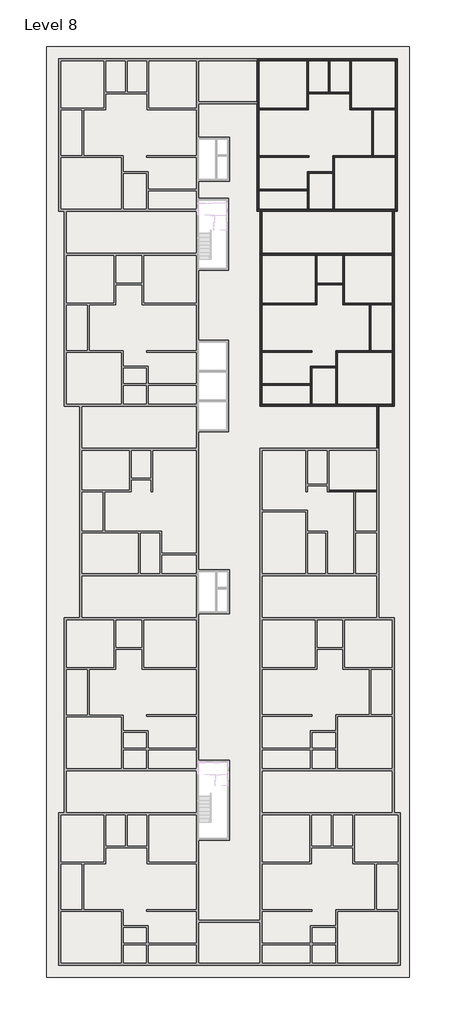
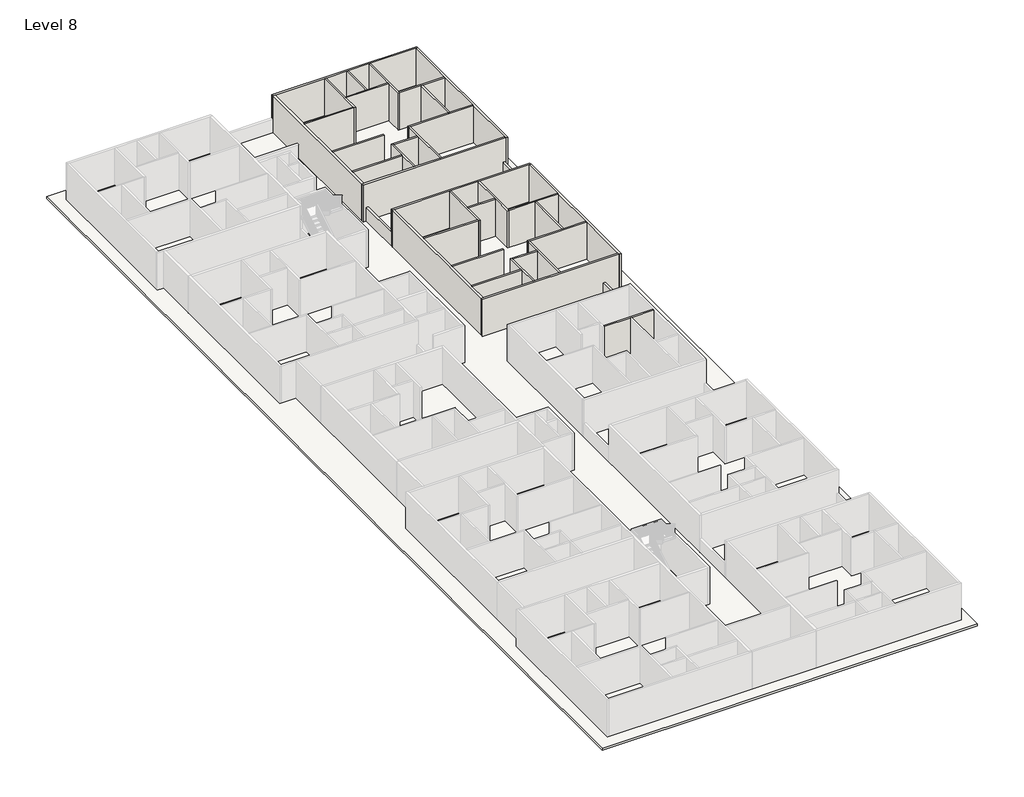
# One storey, part 4 of 8: 37 walls, 1 roof, 1 slab.
"""IFC4 building model written with IfcOpenShell, lengths in millimetres."""

from ifc_helpers import new_model, si_unit, frame, origin, place, context, project, spatial, polyline, outline, extrude, faceted_brep, element, save

model = new_model("IFC4")

# Units and contexts
model_context = context("Model", 3, world=origin())
ifc_project = project(units=[si_unit("LENGTHUNIT", "METRE", prefix="MILLI")], contexts=[model_context])

# Site, building, storey
site = spatial("IfcSite", under=ifc_project)
building = spatial("IfcBuilding", under=site)
storey = spatial("IfcBuildingStorey", under=building, Name="Level 8", Elevation=46570.6172466)

# Roof
placement = place(None, origin())
element("IfcRoof", 1, ObjectType="SLAB", at=placement, inside=storey, context=model_context, shape_type="SweptSolid", body=[
    extrude(outline(polyline([(-15237.9415084, -35021.5344126), (-15237.9415084, 36097.9216096), (12498.9443719, 36097.9216096), (12498.9443719, -35021.5344126), (-15237.9415084, -35021.5344126)]), holes=[polyline([(-3617.4415084, 29152.4900967), (-3617.4415084, 25799.6900967), (-1255.2415084, 25799.6900967), (-1255.2415084, 29152.4900967), (-3617.4415084, 29152.4900967)]), polyline([(-3617.4415084, 24490.1216096), (-3617.4415084, 19003.7216096), (-1331.4415084, 19003.7216096), (-1331.4415084, 24490.1216096), (-3617.4415084, 24490.1216096)]), polyline([(-3617.4415084, 13669.6303368), (-3617.4415084, 6659.2303368), (-1331.4415084, 6659.2303368), (-1331.4415084, 13669.6303368), (-3617.4415084, 13669.6303368)]), polyline([(-3617.4415084, -3882.2751812), (-3617.4415084, -7235.0751812), (-1255.2415084, -7235.0751812), (-1255.2415084, -3882.2751812), (-3617.4415084, -3882.2751812)]), polyline([(-3617.4415084, -18429.9851539), (-3617.4415084, -24525.9851539), (-1229.8415084, -24525.9851539), (-1229.8415084, -18429.9851539), (-3617.4415084, -18429.9851539)])]), frame((0.0, 0.0, 46570.6172466), z_axis=(0.0, 0.0, 1.0), x_axis=(1.0, 0.0, 0.0)), (0.0, 0.0, 1.0), 152.4),
])

# Slab
element("IfcSlab", 2, ObjectType="FLOOR", at=placement, inside=storey, context=model_context, shape_type="SweptSolid", body=[
    extrude(outline(polyline([(-14323.5415084, 35183.5216096), (11584.5443719, 35183.5216096), (11584.5443719, 23499.5216096), (11360.9214687, 23499.5216096), (11360.9214687, 8615.1216096), (10173.4714687, 8615.1216096), (10173.4714687, -7538.7344126), (11360.9214687, -7538.7344126), (11360.9214687, -22423.1344126), (11813.0584916, -22423.1344126), (11813.0584916, -34107.1344126), (11584.5443719, -34107.1344126), (-14323.5415084, -34107.1344126), (-14323.5415084, 35183.5216096)]), holes=[polyline([(-3617.4415084, 29152.4900967), (-3617.4415084, 25799.6900967), (-1255.2415084, 25799.6900967), (-1255.2415084, 29152.4900967), (-3617.4415084, 29152.4900967)]), polyline([(-3617.4415084, 24490.1216096), (-3617.4415084, 19003.7216096), (-1331.4415084, 19003.7216096), (-1331.4415084, 24490.1216096), (-3617.4415084, 24490.1216096)]), polyline([(-3617.4415084, 13669.6303368), (-3617.4415084, 6659.2303368), (-1331.4415084, 6659.2303368), (-1331.4415084, 13669.6303368), (-3617.4415084, 13669.6303368)]), polyline([(-3617.4415084, -3882.2751812), (-3617.4415084, -7235.0751812), (-1255.2415084, -7235.0751812), (-1255.2415084, -3882.2751812), (-3617.4415084, -3882.2751812)]), polyline([(-3617.4415084, -18429.9851539), (-3617.4415084, -24525.9851539), (-1229.8415084, -24525.9851539), (-1229.8415084, -18429.9851539), (-3617.4415084, -18429.9851539)])]), frame((0.0, 0.0, 45961.0172466), z_axis=(0.0, 0.0, 1.0), x_axis=(1.0, 0.0, 0.0)), (0.0, 0.0, 1.0), 609.6),
])

# Walls
element("IfcWall", 3, ObjectType="4.5\"", at=placement, inside=storey, context=model_context, shape_type="Brep", body=[
    faceted_brep([(6363.4714687, 2100.0216096, 46570.6172466), (8282.4584916, 2100.0216096, 46570.6172466), (8396.7584916, 2100.0216096, 46570.6172466), (10021.0714687, 2100.0216096, 46570.6172466), (10021.0714687, 2100.0216096, 49618.6172466), (8396.7584916, 2100.0216096, 49618.6172466), (8282.4584916, 2100.0216096, 49618.6172466), (6363.4714687, 2100.0216096, 49618.6172466), (6363.4714687, 2214.3216096, 46570.6172466), (6363.4714687, 2214.3216096, 49618.6172466), (10021.0714687, 2214.3216096, 49618.6172466), (10021.0714687, 2214.3216096, 46570.6172466)], [[[0, 1, 2, 3, 4, 5, 6, 7]], [[8, 9, 10, 11]], [[3, 2, 1, 0, 8, 11]], [[0, 7, 9, 8]], [[4, 3, 11, 10]], [[7, 6, 5, 4, 10, 9]]]),
])
element("IfcWall", 4, ObjectType="4.5\"", at=placement, inside=storey, context=model_context, shape_type="Brep", body=[
    faceted_brep([(5315.7214687, 20146.7216096, 46570.6172466), (5315.7214687, 16489.1216096, 46570.6172466), (5315.7214687, 16374.8216096, 46570.6172466), (5315.7214687, 16374.8216096, 49618.6172466), (5315.7214687, 16489.1216096, 49618.6172466), (5315.7214687, 20146.7216096, 49618.6172466), (5430.0214687, 20146.7216096, 46570.6172466), (5430.0214687, 20146.7216096, 49618.6172466), (5430.0214687, 18013.1216096, 49618.6172466), (5430.0214687, 17898.8216096, 49618.6172466), (5430.0214687, 16374.8216096, 49618.6172466), (5430.0214687, 16374.8216096, 46570.6172466), (5430.0214687, 17898.8216096, 46570.6172466), (5430.0214687, 18013.1216096, 46570.6172466)], [[[0, 1, 2, 3, 4, 5]], [[6, 7, 8, 9, 10, 11, 12, 13]], [[2, 1, 0, 6, 13, 12, 11]], [[0, 5, 7, 6]], [[3, 2, 11, 10]], [[5, 4, 3, 10, 9, 8, 7]]]),
])
element("IfcWall", 5, ObjectType="4.5\"", at=placement, inside=storey, context=model_context, shape_type="SweptSolid", body=[
    extrude(outline(polyline([(1259.3584916, 16489.1216096), (5315.7214687, 16489.1216096), (5315.7214687, 16374.8216096), (1259.3584916, 16374.8216096), (1259.3584916, 16489.1216096)])), frame((0.0, 0.0, 46570.6172466), z_axis=(0.0, 0.0, 1.0), x_axis=(1.0, 0.0, 0.0)), (0.0, 0.0, 1.0), 3048.0),
])
element("IfcWall", 6, ObjectType="4.5\"", at=placement, inside=storey, context=model_context, shape_type="SweptSolid", body=[
    extrude(outline(polyline([(7436.6214687, 17898.8216096), (5430.0214687, 17898.8216096), (5430.0214687, 18013.1216096), (7436.6214687, 18013.1216096), (7436.6214687, 17898.8216096)])), frame((0.0, 0.0, 46570.6172466), z_axis=(0.0, 0.0, 1.0), x_axis=(1.0, 0.0, 0.0)), (0.0, 0.0, 1.0), 3048.0),
])
element("IfcWall", 7, ObjectType="4.5\"", at=placement, inside=storey, context=model_context, shape_type="Brep", body=[
    faceted_brep([(7436.6214687, 20146.7216096, 46570.6172466), (7436.6214687, 18013.1216096, 46570.6172466), (7436.6214687, 17898.8216096, 46570.6172466), (7436.6214687, 16374.8216096, 46570.6172466), (7436.6214687, 16374.8216096, 49618.6172466), (7436.6214687, 17898.8216096, 49618.6172466), (7436.6214687, 18013.1216096, 49618.6172466), (7436.6214687, 20146.7216096, 49618.6172466), (7550.9214687, 20146.7216096, 46570.6172466), (7550.9214687, 20146.7216096, 49618.6172466), (7550.9214687, 16489.1216096, 49618.6172466), (7550.9214687, 16374.8216096, 49618.6172466), (7550.9214687, 16374.8216096, 46570.6172466), (7550.9214687, 16489.1216096, 46570.6172466)], [[[0, 1, 2, 3, 4, 5, 6, 7]], [[8, 9, 10, 11, 12, 13]], [[3, 2, 1, 0, 8, 13, 12]], [[0, 7, 9, 8]], [[4, 3, 12, 11]], [[7, 6, 5, 4, 11, 10, 9]]]),
])
element("IfcWall", 8, ObjectType="4.5\"", at=placement, inside=storey, context=model_context, shape_type="Brep", body=[
    faceted_brep([(7550.9214687, 16374.8216096, 46570.6172466), (9469.9084916, 16374.8216096, 46570.6172466), (9584.2084916, 16374.8216096, 46570.6172466), (11208.5214687, 16374.8216096, 46570.6172466), (11208.5214687, 16374.8216096, 49618.6172466), (9584.2084916, 16374.8216096, 49618.6172466), (9469.9084916, 16374.8216096, 49618.6172466), (7550.9214687, 16374.8216096, 49618.6172466), (7550.9214687, 16489.1216096, 46570.6172466), (7550.9214687, 16489.1216096, 49618.6172466), (11208.5214687, 16489.1216096, 49618.6172466), (11208.5214687, 16489.1216096, 46570.6172466)], [[[0, 1, 2, 3, 4, 5, 6, 7]], [[8, 9, 10, 11]], [[3, 2, 1, 0, 8, 11]], [[0, 7, 9, 8]], [[4, 3, 11, 10]], [[7, 6, 5, 4, 10, 9]]]),
])
element("IfcWall", 9, ObjectType="4.5\"", at=placement, inside=storey, context=model_context, shape_type="SweptSolid", body=[
    extrude(outline(polyline([(9469.9084916, 12869.6216096), (9469.9084916, 16374.8216096), (9584.2084916, 16374.8216096), (9584.2084916, 12869.6216096), (9469.9084916, 12869.6216096)])), frame((0.0, 0.0, 46570.6172466), z_axis=(0.0, 0.0, 1.0), x_axis=(1.0, 0.0, 0.0)), (0.0, 0.0, 1.0), 3048.0),
])
element("IfcWall", 10, ObjectType="4.5\"", at=placement, inside=storey, context=model_context, shape_type="Brep", body=[
    faceted_brep([(11208.5214687, 12869.6216096, 46570.6172466), (9584.2084916, 12869.6216096, 46570.6172466), (9469.9084916, 12869.6216096, 46570.6172466), (6885.4584916, 12869.6216096, 46570.6172466), (6885.4584916, 12869.6216096, 49618.6172466), (9469.9084916, 12869.6216096, 49618.6172466), (9584.2084916, 12869.6216096, 49618.6172466), (11208.5214687, 12869.6216096, 49618.6172466), (11208.5214687, 12755.3216096, 46570.6172466), (11208.5214687, 12755.3216096, 49618.6172466), (6999.7584916, 12755.3216096, 49618.6172466), (6885.4584916, 12755.3216096, 49618.6172466), (6885.4584916, 12755.3216096, 46570.6172466), (6999.7584916, 12755.3216096, 46570.6172466)], [[[0, 1, 2, 3, 4, 5, 6, 7]], [[8, 9, 10, 11, 12, 13]], [[3, 2, 1, 0, 8, 13, 12]], [[0, 7, 9, 8]], [[4, 3, 12, 11]], [[7, 6, 5, 4, 11, 10, 9]]]),
])
element("IfcWall", 11, ObjectType="4.5\"", at=placement, inside=storey, context=model_context, shape_type="Brep", body=[
    faceted_brep([(6885.4584916, 12755.3216096, 46570.6172466), (6885.4584916, 11663.1216096, 46570.6172466), (6885.4584916, 11548.8216096, 46570.6172466), (6885.4584916, 8767.5216096, 46570.6172466), (6885.4584916, 8767.5216096, 49618.6172466), (6885.4584916, 11548.8216096, 49618.6172466), (6885.4584916, 11663.1216096, 49618.6172466), (6885.4584916, 12755.3216096, 49618.6172466), (6999.7584916, 12755.3216096, 46570.6172466), (6999.7584916, 12755.3216096, 49618.6172466), (6999.7584916, 8767.5216096, 49618.6172466), (6999.7584916, 8767.5216096, 46570.6172466)], [[[0, 1, 2, 3, 4, 5, 6, 7]], [[8, 9, 10, 11]], [[3, 2, 1, 0, 8, 11]], [[0, 7, 9, 8]], [[4, 3, 11, 10]], [[7, 6, 5, 4, 10, 9]]]),
])
element("IfcWall", 12, ObjectType="4.5\"", at=placement, inside=storey, context=model_context, shape_type="Brep", body=[
    faceted_brep([(5056.6584916, 8767.5216096, 46570.6172466), (5056.6584916, 11548.8216096, 46570.6172466), (5056.6584916, 11663.1216096, 46570.6172466), (5056.6584916, 11663.1216096, 49618.6172466), (5056.6584916, 11548.8216096, 49618.6172466), (5056.6584916, 8767.5216096, 49618.6172466), (4942.3584916, 8767.5216096, 46570.6172466), (4942.3584916, 8767.5216096, 49618.6172466), (4942.3584916, 10215.3216096, 49618.6172466), (4942.3584916, 10329.6216096, 49618.6172466), (4942.3584916, 11663.1216096, 49618.6172466), (4942.3584916, 11663.1216096, 46570.6172466), (4942.3584916, 10329.6216096, 46570.6172466), (4942.3584916, 10215.3216096, 46570.6172466)], [[[0, 1, 2, 3, 4, 5]], [[6, 7, 8, 9, 10, 11, 12, 13]], [[2, 1, 0, 6, 13, 12, 11]], [[0, 5, 7, 6]], [[3, 2, 11, 10]], [[5, 4, 3, 10, 9, 8, 7]]]),
])
element("IfcWall", 13, ObjectType="4.5\"", at=placement, inside=storey, context=model_context, shape_type="SweptSolid", body=[
    extrude(outline(polyline([(6885.4584916, 11548.8216096), (5056.6584916, 11548.8216096), (5056.6584916, 11663.1216096), (6885.4584916, 11663.1216096), (6885.4584916, 11548.8216096)])), frame((0.0, 0.0, 46570.6172466), z_axis=(0.0, 0.0, 1.0), x_axis=(1.0, 0.0, 0.0)), (0.0, 0.0, 1.0), 3048.0),
])
element("IfcWall", 14, ObjectType="4.5\"", at=placement, inside=storey, context=model_context, shape_type="SweptSolid", body=[
    extrude(outline(polyline([(4942.3584916, 10215.3216096), (1259.3584916, 10215.3216096), (1259.3584916, 10329.6216096), (4942.3584916, 10329.6216096), (4942.3584916, 10215.3216096)])), frame((0.0, 0.0, 46570.6172466), z_axis=(0.0, 0.0, 1.0), x_axis=(1.0, 0.0, 0.0)), (0.0, 0.0, 1.0), 3048.0),
])
element("IfcWall", 15, ObjectType="4.5\"", at=placement, inside=storey, context=model_context, shape_type="SweptSolid", body=[
    extrude(outline(polyline([(5056.6584916, 12755.3216096), (1259.3584916, 12755.3216096), (1259.3584916, 12869.6216096), (5056.6584916, 12869.6216096), (5056.6584916, 12755.3216096)])), frame((0.0, 0.0, 46570.6172466), z_axis=(0.0, 0.0, 1.0), x_axis=(1.0, 0.0, 0.0)), (0.0, 0.0, 1.0), 3048.0),
])
element("IfcWall", 16, ObjectType="4.5\"", at=placement, inside=storey, context=model_context, shape_type="Brep", body=[
    faceted_brep([(4688.4443719, 35031.1216096, 46570.6172466), (4688.4443719, 31373.5216096, 46570.6172466), (4688.4443719, 31259.2216096, 46570.6172466), (4688.4443719, 31259.2216096, 49618.6172466), (4688.4443719, 31373.5216096, 49618.6172466), (4688.4443719, 35031.1216096, 49618.6172466), (4802.7443719, 35031.1216096, 46570.6172466), (4802.7443719, 35031.1216096, 49618.6172466), (4802.7443719, 32592.7216096, 49618.6172466), (4802.7443719, 32478.4216096, 49618.6172466), (4802.7443719, 31259.2216096, 49618.6172466), (4802.7443719, 31259.2216096, 46570.6172466), (4802.7443719, 32478.4216096, 46570.6172466), (4802.7443719, 32592.7216096, 46570.6172466)], [[[0, 1, 2, 3, 4, 5]], [[6, 7, 8, 9, 10, 11, 12, 13]], [[2, 1, 0, 6, 13, 12, 11]], [[0, 5, 7, 6]], [[3, 2, 11, 10]], [[5, 4, 3, 10, 9, 8, 7]]]),
])
element("IfcWall", 17, ObjectType="4.5\"", at=placement, inside=storey, context=model_context, shape_type="SweptSolid", body=[
    extrude(outline(polyline([(1030.8443719, 31373.5216096), (4688.4443719, 31373.5216096), (4688.4443719, 31259.2216096), (1030.8443719, 31259.2216096), (1030.8443719, 31373.5216096)])), frame((0.0, 0.0, 46570.6172466), z_axis=(0.0, 0.0, 1.0), x_axis=(1.0, 0.0, 0.0)), (0.0, 0.0, 1.0), 3048.0),
])
element("IfcWall", 18, ObjectType="4.5\"", at=placement, inside=storey, context=model_context, shape_type="Brep", body=[
    faceted_brep([(4802.7443719, 32478.4216096, 46570.6172466), (7965.0443719, 32478.4216096, 46570.6172466), (7965.0443719, 32478.4216096, 49618.6172466), (4802.7443719, 32478.4216096, 49618.6172466), (4802.7443719, 32592.7216096, 46570.6172466), (4802.7443719, 32592.7216096, 49618.6172466), (6326.7443719, 32592.7216096, 49618.6172466), (6441.0443719, 32592.7216096, 49618.6172466), (7965.0443719, 32592.7216096, 49618.6172466), (7965.0443719, 32592.7216096, 46570.6172466), (6441.0443719, 32592.7216096, 46570.6172466), (6326.7443719, 32592.7216096, 46570.6172466)], [[[0, 1, 2, 3]], [[4, 5, 6, 7, 8, 9, 10, 11]], [[1, 0, 4, 11, 10, 9]], [[0, 3, 5, 4]], [[2, 1, 9, 8]], [[3, 2, 8, 7, 6, 5]]]),
])
element("IfcWall", 19, ObjectType="4.5\"", at=placement, inside=storey, context=model_context, shape_type="SweptSolid", body=[
    extrude(outline(polyline([(6326.7443719, 32592.7216096), (6326.7443719, 35031.1216096), (6441.0443719, 35031.1216096), (6441.0443719, 32592.7216096), (6326.7443719, 32592.7216096)])), frame((0.0, 0.0, 46570.6172466), z_axis=(0.0, 0.0, 1.0), x_axis=(1.0, 0.0, 0.0)), (0.0, 0.0, 1.0), 3048.0),
])
element("IfcWall", 20, ObjectType="4.5\"", at=placement, inside=storey, context=model_context, shape_type="Brep", body=[
    faceted_brep([(7965.0443719, 35031.1216096, 46570.6172466), (7965.0443719, 32592.7216096, 46570.6172466), (7965.0443719, 32478.4216096, 46570.6172466), (7965.0443719, 31259.2216096, 46570.6172466), (7965.0443719, 31259.2216096, 49618.6172466), (7965.0443719, 32478.4216096, 49618.6172466), (7965.0443719, 32592.7216096, 49618.6172466), (7965.0443719, 35031.1216096, 49618.6172466), (8079.3443719, 35031.1216096, 46570.6172466), (8079.3443719, 35031.1216096, 49618.6172466), (8079.3443719, 31373.5216096, 49618.6172466), (8079.3443719, 31259.2216096, 49618.6172466), (8079.3443719, 31259.2216096, 46570.6172466), (8079.3443719, 31373.5216096, 46570.6172466)], [[[0, 1, 2, 3, 4, 5, 6, 7]], [[8, 9, 10, 11, 12, 13]], [[3, 2, 1, 0, 8, 13, 12]], [[0, 7, 9, 8]], [[4, 3, 12, 11]], [[7, 6, 5, 4, 11, 10, 9]]]),
])
element("IfcWall", 21, ObjectType="4.5\"", at=placement, inside=storey, context=model_context, shape_type="Brep", body=[
    faceted_brep([(8079.3443719, 31259.2216096, 46570.6172466), (9641.4443719, 31259.2216096, 46570.6172466), (9755.7443719, 31259.2216096, 46570.6172466), (11432.1443719, 31259.2216096, 46570.6172466), (11432.1443719, 31259.2216096, 49618.6172466), (9755.7443719, 31259.2216096, 49618.6172466), (9641.4443719, 31259.2216096, 49618.6172466), (8079.3443719, 31259.2216096, 49618.6172466), (8079.3443719, 31373.5216096, 46570.6172466), (8079.3443719, 31373.5216096, 49618.6172466), (11432.1443719, 31373.5216096, 49618.6172466), (11432.1443719, 31373.5216096, 46570.6172466)], [[[0, 1, 2, 3, 4, 5, 6, 7]], [[8, 9, 10, 11]], [[3, 2, 1, 0, 8, 11]], [[0, 7, 9, 8]], [[4, 3, 11, 10]], [[7, 6, 5, 4, 10, 9]]]),
])
element("IfcWall", 22, ObjectType="4.5\"", at=placement, inside=storey, context=model_context, shape_type="SweptSolid", body=[
    extrude(outline(polyline([(9641.4443719, 27754.0216096), (9641.4443719, 31259.2216096), (9755.7443719, 31259.2216096), (9755.7443719, 27754.0216096), (9641.4443719, 27754.0216096)])), frame((0.0, 0.0, 46570.6172466), z_axis=(0.0, 0.0, 1.0), x_axis=(1.0, 0.0, 0.0)), (0.0, 0.0, 1.0), 3048.0),
])
element("IfcWall", 23, ObjectType="4.5\"", at=placement, inside=storey, context=model_context, shape_type="Brep", body=[
    faceted_brep([(11432.1443719, 27754.0216096, 46570.6172466), (9755.7443719, 27754.0216096, 46570.6172466), (9641.4443719, 27754.0216096, 46570.6172466), (6656.9443719, 27754.0216096, 46570.6172466), (6656.9443719, 27754.0216096, 49618.6172466), (9641.4443719, 27754.0216096, 49618.6172466), (9755.7443719, 27754.0216096, 49618.6172466), (11432.1443719, 27754.0216096, 49618.6172466), (11432.1443719, 27639.7216096, 46570.6172466), (11432.1443719, 27639.7216096, 49618.6172466), (6771.2443719, 27639.7216096, 49618.6172466), (6656.9443719, 27639.7216096, 49618.6172466), (6656.9443719, 27639.7216096, 46570.6172466), (6771.2443719, 27639.7216096, 46570.6172466)], [[[0, 1, 2, 3, 4, 5, 6, 7]], [[8, 9, 10, 11, 12, 13]], [[3, 2, 1, 0, 8, 13, 12]], [[0, 7, 9, 8]], [[4, 3, 12, 11]], [[7, 6, 5, 4, 11, 10, 9]]]),
])
element("IfcWall", 24, ObjectType="4.5\"", at=placement, inside=storey, context=model_context, shape_type="Brep", body=[
    faceted_brep([(6656.9443719, 27639.7216096, 46570.6172466), (6656.9443719, 26547.5216096, 46570.6172466), (6656.9443719, 26433.2216096, 46570.6172466), (6656.9443719, 23651.9216096, 46570.6172466), (6656.9443719, 23651.9216096, 49618.6172466), (6656.9443719, 26433.2216096, 49618.6172466), (6656.9443719, 26547.5216096, 49618.6172466), (6656.9443719, 27639.7216096, 49618.6172466), (6771.2443719, 27639.7216096, 46570.6172466), (6771.2443719, 27639.7216096, 49618.6172466), (6771.2443719, 23651.9216096, 49618.6172466), (6771.2443719, 23651.9216096, 46570.6172466)], [[[0, 1, 2, 3, 4, 5, 6, 7]], [[8, 9, 10, 11]], [[3, 2, 1, 0, 8, 11]], [[0, 7, 9, 8]], [[4, 3, 11, 10]], [[7, 6, 5, 4, 10, 9]]]),
])
element("IfcWall", 25, ObjectType="4.5\"", at=placement, inside=storey, context=model_context, shape_type="SweptSolid", body=[
    extrude(outline(polyline([(4713.8443719, 25099.7216096), (1030.8443719, 25099.7216096), (1030.8443719, 25214.0216096), (4713.8443719, 25214.0216096), (4713.8443719, 25099.7216096)])), frame((0.0, 0.0, 46570.6172466), z_axis=(0.0, 0.0, 1.0), x_axis=(1.0, 0.0, 0.0)), (0.0, 0.0, 1.0), 3048.0),
])
element("IfcWall", 26, ObjectType="4.5\"", at=placement, inside=storey, context=model_context, shape_type="Brep", body=[
    faceted_brep([(4828.1443719, 23651.9216096, 46570.6172466), (4828.1443719, 26433.2216096, 46570.6172466), (4828.1443719, 26547.5216096, 46570.6172466), (4828.1443719, 26547.5216096, 49618.6172466), (4828.1443719, 26433.2216096, 49618.6172466), (4828.1443719, 23651.9216096, 49618.6172466), (4713.8443719, 23651.9216096, 46570.6172466), (4713.8443719, 23651.9216096, 49618.6172466), (4713.8443719, 25099.7216096, 49618.6172466), (4713.8443719, 25214.0216096, 49618.6172466), (4713.8443719, 26547.5216096, 49618.6172466), (4713.8443719, 26547.5216096, 46570.6172466), (4713.8443719, 25214.0216096, 46570.6172466), (4713.8443719, 25099.7216096, 46570.6172466)], [[[0, 1, 2, 3, 4, 5]], [[6, 7, 8, 9, 10, 11, 12, 13]], [[2, 1, 0, 6, 13, 12, 11]], [[0, 5, 7, 6]], [[3, 2, 11, 10]], [[5, 4, 3, 10, 9, 8, 7]]]),
])
element("IfcWall", 27, ObjectType="4.5\"", at=placement, inside=storey, context=model_context, shape_type="SweptSolid", body=[
    extrude(outline(polyline([(6656.9443719, 26433.2216096), (4828.1443719, 26433.2216096), (4828.1443719, 26547.5216096), (6656.9443719, 26547.5216096), (6656.9443719, 26433.2216096)])), frame((0.0, 0.0, 46570.6172466), z_axis=(0.0, 0.0, 1.0), x_axis=(1.0, 0.0, 0.0)), (0.0, 0.0, 1.0), 3048.0),
])
element("IfcWall", 28, ObjectType="4.5\"", at=placement, inside=storey, context=model_context, shape_type="SweptSolid", body=[
    extrude(outline(polyline([(4828.1443719, 27639.7216096), (1030.8443719, 27639.7216096), (1030.8443719, 27754.0216096), (4828.1443719, 27754.0216096), (4828.1443719, 27639.7216096)])), frame((0.0, 0.0, 46570.6172466), z_axis=(0.0, 0.0, 1.0), x_axis=(1.0, 0.0, 0.0)), (0.0, 0.0, 1.0), 3048.0),
])
element("IfcWall", 29, ObjectType="6\"", at=placement, inside=storey, context=model_context, shape_type="Brep", body=[
    faceted_brep([(1106.9584916, 20146.7216096, 49618.6172466), (1106.9584916, 20146.7216096, 46570.6172466), (1259.3584916, 20146.7216096, 46570.6172466), (5315.7214687, 20146.7216096, 46570.6172466), (5430.0214687, 20146.7216096, 46570.6172466), (7436.6214687, 20146.7216096, 46570.6172466), (7550.9214687, 20146.7216096, 46570.6172466), (11208.5214687, 20146.7216096, 46570.6172466), (11360.9214687, 20146.7216096, 46570.6172466), (11360.9214687, 20146.7216096, 49618.6172466), (11208.5214687, 20146.7216096, 49618.6172466), (7550.9214687, 20146.7216096, 49618.6172466), (7436.6214687, 20146.7216096, 49618.6172466), (5430.0214687, 20146.7216096, 49618.6172466), (5315.7214687, 20146.7216096, 49618.6172466), (1259.3584916, 20146.7216096, 49618.6172466), (1106.9584916, 20299.1216096, 46570.6172466), (1106.9584916, 20299.1216096, 47789.8172466), (1106.9584916, 20299.1216096, 49618.6172466), (11360.9214687, 20299.1216096, 49618.6172466), (11360.9214687, 20299.1216096, 47789.8172466), (11360.9214687, 20299.1216096, 46570.6172466), (11208.5214687, 20299.1216096, 46570.6172466), (1259.3584916, 20299.1216096, 46570.6172466)], [[[0, 1, 2, 3, 4, 5, 6, 7, 8, 9, 10, 11, 12, 13, 14, 15]], [[16, 17, 18, 19, 20, 21, 22, 23]], [[8, 7, 6, 5, 4, 3, 2, 1, 16, 23, 22, 21]], [[0, 18, 17, 16, 1]], [[8, 21, 20, 19, 9]], [[0, 15, 14, 13, 12, 11, 10, 9, 19, 18]]]),
])
element("IfcWall", 30, ObjectType="6\"", at=placement, inside=storey, context=model_context, shape_type="Brep", body=[
    faceted_brep([(11208.5214687, 20146.7216096, 49618.6172466), (11208.5214687, 20146.7216096, 46570.6172466), (11208.5214687, 16489.1216096, 46570.6172466), (11208.5214687, 16374.8216096, 46570.6172466), (11208.5214687, 12869.6216096, 46570.6172466), (11208.5214687, 12755.3216096, 46570.6172466), (11208.5214687, 8767.5216096, 46570.6172466), (11208.5214687, 8615.1216096, 46570.6172466), (11208.5214687, 8615.1216096, 49618.6172466), (11208.5214687, 8767.5216096, 49618.6172466), (11208.5214687, 12755.3216096, 49618.6172466), (11208.5214687, 12869.6216096, 49618.6172466), (11208.5214687, 16374.8216096, 49618.6172466), (11208.5214687, 16489.1216096, 49618.6172466), (11360.9214687, 20146.7216096, 46570.6172466), (11360.9214687, 20146.7216096, 49618.6172466), (11360.9214687, 8615.1216096, 49618.6172466), (11360.9214687, 8615.1216096, 46570.6172466)], [[[0, 1, 2, 3, 4, 5, 6, 7, 8, 9, 10, 11, 12, 13]], [[14, 15, 16, 17]], [[7, 6, 5, 4, 3, 2, 1, 14, 17]], [[8, 7, 17, 16]], [[0, 15, 14, 1]], [[0, 13, 12, 11, 10, 9, 8, 16, 15]]]),
])
element("IfcWall", 31, ObjectType="6\"", at=placement, inside=storey, context=model_context, shape_type="Brep", body=[
    faceted_brep([(11208.5214687, 8767.5216096, 46570.6172466), (6999.7584916, 8767.5216096, 46570.6172466), (6885.4584916, 8767.5216096, 46570.6172466), (5056.6584916, 8767.5216096, 46570.6172466), (4942.3584916, 8767.5216096, 46570.6172466), (1259.3584916, 8767.5216096, 46570.6172466), (1106.9584916, 8767.5216096, 46570.6172466), (1106.9584916, 8767.5216096, 49618.6172466), (1259.3584916, 8767.5216096, 49618.6172466), (4942.3584916, 8767.5216096, 49618.6172466), (5056.6584916, 8767.5216096, 49618.6172466), (6885.4584916, 8767.5216096, 49618.6172466), (6999.7584916, 8767.5216096, 49618.6172466), (11208.5214687, 8767.5216096, 49618.6172466), (11208.5214687, 8615.1216096, 46570.6172466), (11208.5214687, 8615.1216096, 49618.6172466), (1106.9584916, 8615.1216096, 49618.6172466), (1106.9584916, 8615.1216096, 46570.6172466), (10021.0714687, 8615.1216096, 46570.6172466), (10173.4714687, 8615.1216096, 46570.6172466)], [[[0, 1, 2, 3, 4, 5, 6, 7, 8, 9, 10, 11, 12, 13]], [[14, 15, 16, 17, 18, 19]], [[6, 5, 4, 3, 2, 1, 0, 14, 19, 18, 17]], [[0, 13, 15, 14]], [[7, 6, 17, 16]], [[13, 12, 11, 10, 9, 8, 7, 16, 15]]]),
])
element("IfcWall", 32, ObjectType="6\"", at=placement, inside=storey, context=model_context, shape_type="Brep", body=[
    faceted_brep([(1259.3584916, 8767.5216096, 46570.6172466), (1259.3584916, 10215.3216096, 46570.6172466), (1259.3584916, 10329.6216096, 46570.6172466), (1259.3584916, 12755.3216096, 46570.6172466), (1259.3584916, 12869.6216096, 46570.6172466), (1259.3584916, 16374.8216096, 46570.6172466), (1259.3584916, 16489.1216096, 46570.6172466), (1259.3584916, 20146.7216096, 46570.6172466), (1259.3584916, 20146.7216096, 49618.6172466), (1259.3584916, 16489.1216096, 49618.6172466), (1259.3584916, 16374.8216096, 49618.6172466), (1259.3584916, 12869.6216096, 49618.6172466), (1259.3584916, 12755.3216096, 49618.6172466), (1259.3584916, 10329.6216096, 49618.6172466), (1259.3584916, 10215.3216096, 49618.6172466), (1259.3584916, 8767.5216096, 49618.6172466), (1106.9584916, 8767.5216096, 46570.6172466), (1106.9584916, 8767.5216096, 49618.6172466), (1106.9584916, 20146.7216096, 49618.6172466), (1106.9584916, 20146.7216096, 46570.6172466)], [[[0, 1, 2, 3, 4, 5, 6, 7, 8, 9, 10, 11, 12, 13, 14, 15]], [[16, 17, 18, 19]], [[7, 6, 5, 4, 3, 2, 1, 0, 16, 19]], [[0, 15, 17, 16]], [[7, 19, 18, 8]], [[15, 14, 13, 12, 11, 10, 9, 8, 18, 17]]]),
])
element("IfcWall", 33, ObjectType="6\"", at=placement, inside=storey, context=model_context, shape_type="Brep", body=[
    faceted_brep([(878.4443719, 35031.1216096, 49618.6172466), (878.4443719, 35031.1216096, 46570.6172466), (1030.8443719, 35031.1216096, 46570.6172466), (4688.4443719, 35031.1216096, 46570.6172466), (4802.7443719, 35031.1216096, 46570.6172466), (6326.7443719, 35031.1216096, 46570.6172466), (6441.0443719, 35031.1216096, 46570.6172466), (7965.0443719, 35031.1216096, 46570.6172466), (8079.3443719, 35031.1216096, 46570.6172466), (11432.1443719, 35031.1216096, 46570.6172466), (11584.5443719, 35031.1216096, 46570.6172466), (11584.5443719, 35031.1216096, 49618.6172466), (11432.1443719, 35031.1216096, 49618.6172466), (8079.3443719, 35031.1216096, 49618.6172466), (7965.0443719, 35031.1216096, 49618.6172466), (6441.0443719, 35031.1216096, 49618.6172466), (6326.7443719, 35031.1216096, 49618.6172466), (4802.7443719, 35031.1216096, 49618.6172466), (4688.4443719, 35031.1216096, 49618.6172466), (1030.8443719, 35031.1216096, 49618.6172466), (878.4443719, 35183.5216096, 46570.6172466), (878.4443719, 35183.5216096, 49618.6172466), (11584.5443719, 35183.5216096, 49618.6172466), (11584.5443719, 35183.5216096, 46570.6172466)], [[[0, 1, 2, 3, 4, 5, 6, 7, 8, 9, 10, 11, 12, 13, 14, 15, 16, 17, 18, 19]], [[20, 21, 22, 23]], [[10, 9, 8, 7, 6, 5, 4, 3, 2, 1, 20, 23]], [[11, 10, 23, 22]], [[0, 21, 20, 1]], [[0, 19, 18, 17, 16, 15, 14, 13, 12, 11, 22, 21]]]),
])
element("IfcWall", 34, ObjectType="6\"", at=placement, inside=storey, context=model_context, shape_type="Brep", body=[
    faceted_brep([(11432.1443719, 35031.1216096, 46570.6172466), (11432.1443719, 31373.5216096, 46570.6172466), (11432.1443719, 31259.2216096, 46570.6172466), (11432.1443719, 27754.0216096, 46570.6172466), (11432.1443719, 27639.7216096, 46570.6172466), (11432.1443719, 23651.9216096, 46570.6172466), (11432.1443719, 23499.5216096, 46570.6172466), (11432.1443719, 23499.5216096, 49618.6172466), (11432.1443719, 23651.9216096, 49618.6172466), (11432.1443719, 27639.7216096, 49618.6172466), (11432.1443719, 27754.0216096, 49618.6172466), (11432.1443719, 31259.2216096, 49618.6172466), (11432.1443719, 31373.5216096, 49618.6172466), (11432.1443719, 35031.1216096, 49618.6172466), (11584.5443719, 35031.1216096, 46570.6172466), (11584.5443719, 35031.1216096, 49618.6172466), (11584.5443719, 23499.5216096, 49618.6172466), (11584.5443719, 23499.5216096, 46570.6172466)], [[[0, 1, 2, 3, 4, 5, 6, 7, 8, 9, 10, 11, 12, 13]], [[14, 15, 16, 17]], [[6, 5, 4, 3, 2, 1, 0, 14, 17]], [[0, 13, 15, 14]], [[7, 6, 17, 16]], [[13, 12, 11, 10, 9, 8, 7, 16, 15]]]),
])
element("IfcWall", 35, ObjectType="6\"", at=placement, inside=storey, context=model_context, shape_type="Brep", body=[
    faceted_brep([(11432.1443719, 23651.9216096, 46570.6172466), (6771.2443719, 23651.9216096, 46570.6172466), (6656.9443719, 23651.9216096, 46570.6172466), (4828.1443719, 23651.9216096, 46570.6172466), (4713.8443719, 23651.9216096, 46570.6172466), (1030.8443719, 23651.9216096, 46570.6172466), (878.4443719, 23651.9216096, 46570.6172466), (878.4443719, 23651.9216096, 49618.6172466), (1030.8443719, 23651.9216096, 49618.6172466), (4713.8443719, 23651.9216096, 49618.6172466), (4828.1443719, 23651.9216096, 49618.6172466), (6656.9443719, 23651.9216096, 49618.6172466), (6771.2443719, 23651.9216096, 49618.6172466), (11432.1443719, 23651.9216096, 49618.6172466), (11432.1443719, 23499.5216096, 46570.6172466), (11432.1443719, 23499.5216096, 49618.6172466), (878.4443719, 23499.5216096, 49618.6172466), (878.4443719, 23499.5216096, 46570.6172466), (1106.9584916, 23499.5216096, 46570.6172466), (1259.3584916, 23499.5216096, 46570.6172466), (11208.5214687, 23499.5216096, 46570.6172466), (11360.9214687, 23499.5216096, 46570.6172466)], [[[0, 1, 2, 3, 4, 5, 6, 7, 8, 9, 10, 11, 12, 13]], [[14, 15, 16, 17, 18, 19, 20, 21]], [[6, 5, 4, 3, 2, 1, 0, 14, 21, 20, 19, 18, 17]], [[0, 13, 15, 14]], [[7, 6, 17, 16]], [[13, 12, 11, 10, 9, 8, 7, 16, 15]]]),
])
element("IfcWall", 36, ObjectType="6\"", at=placement, inside=storey, context=model_context, shape_type="Brep", body=[
    faceted_brep([(1030.8443719, 23651.9216096, 46570.6172466), (1030.8443719, 25099.7216096, 46570.6172466), (1030.8443719, 25214.0216096, 46570.6172466), (1030.8443719, 27639.7216096, 46570.6172466), (1030.8443719, 27754.0216096, 46570.6172466), (1030.8443719, 31259.2216096, 46570.6172466), (1030.8443719, 31373.5216096, 46570.6172466), (1030.8443719, 35031.1216096, 46570.6172466), (1030.8443719, 35031.1216096, 49618.6172466), (1030.8443719, 31373.5216096, 49618.6172466), (1030.8443719, 31259.2216096, 49618.6172466), (1030.8443719, 27754.0216096, 49618.6172466), (1030.8443719, 27639.7216096, 49618.6172466), (1030.8443719, 25214.0216096, 49618.6172466), (1030.8443719, 25099.7216096, 49618.6172466), (1030.8443719, 23651.9216096, 49618.6172466), (878.4443719, 23651.9216096, 46570.6172466), (878.4443719, 23651.9216096, 49618.6172466), (878.4443719, 35031.1216096, 49618.6172466), (878.4443719, 35031.1216096, 46570.6172466), (878.4443719, 31897.3197155, 46570.6172466), (878.4443719, 31744.9197155, 46570.6172466)], [[[0, 1, 2, 3, 4, 5, 6, 7, 8, 9, 10, 11, 12, 13, 14, 15]], [[16, 17, 18, 19, 20, 21]], [[7, 6, 5, 4, 3, 2, 1, 0, 16, 21, 20, 19]], [[0, 15, 17, 16]], [[7, 19, 18, 8]], [[15, 14, 13, 12, 11, 10, 9, 8, 18, 17]]]),
])
element("IfcWall", 37, ObjectType="6\" 2", at=placement, inside=storey, context=model_context, shape_type="SweptSolid", body=[
    extrude(outline(polyline([(1106.9584916, 20299.1216096), (1106.9584916, 23499.5216096), (1259.3584916, 23499.5216096), (1259.3584916, 20299.1216096), (1106.9584916, 20299.1216096)])), frame((0.0, 0.0, 46570.6172466), z_axis=(0.0, 0.0, 1.0), x_axis=(1.0, 0.0, 0.0)), (0.0, 0.0, 1.0), 1219.2),
])
element("IfcWall", 38, ObjectType="6\" 2", at=placement, inside=storey, context=model_context, shape_type="SweptSolid", body=[
    extrude(outline(polyline([(11208.5214687, 20299.1216096), (11208.5214687, 23499.5216096), (11360.9214687, 23499.5216096), (11360.9214687, 20299.1216096), (11208.5214687, 20299.1216096)])), frame((0.0, 0.0, 46570.6172466), z_axis=(0.0, 0.0, 1.0), x_axis=(1.0, 0.0, 0.0)), (0.0, 0.0, 1.0), 1219.2),
])
element("IfcWall", 39, ObjectType="6\" 2", at=placement, inside=storey, context=model_context, shape_type="SweptSolid", body=[
    extrude(outline(polyline([(10021.0714687, 5414.7216096), (10021.0714687, 8615.1216096), (10173.4714687, 8615.1216096), (10173.4714687, 5414.7216096), (10021.0714687, 5414.7216096)])), frame((0.0, 0.0, 46570.6172466), z_axis=(0.0, 0.0, 1.0), x_axis=(1.0, 0.0, 0.0)), (0.0, 0.0, 1.0), 1219.2),
])

save(model, "model.ifc")

# Revit data of these elements
# Type "SLAB"
#   Assembly Code = "B1020"
#   Layers, outside or top first: 0' - 6" "Damp-proofing" (function 1)
# Type "FLOOR"
#   Assembly Code = "B1010"
#   Function = 0
#   Layers, outside or top first: 2' - 0" "Tile, Porcelain, 4in" (function 1)
# Type "4.5\""
#   Assembly Code = "B2010"
#   Layers, outside or top first: 0' - 4 1/2" "WALLS" (function 1)
# Type "6\""
#   Assembly Code = "B2010"
#   Layers, outside or top first: 0' - 6" "WALLS" (function 1)
# Type "6\" 2"
#   Assembly Code = "B2010"
#   Layers, outside or top first: 0' - 6" "4'" (function 1)
# Element 1 (IfcRoof, "SLAB")
#   built-in parameter 1001705 = 153.291 (stored number, unit not read)
#   built-in parameter 1001710 = 33615
#   Phase Created = New Construction
#   Materials on its faces: "Damp-proofing"
# Element 2 (IfcSlab, "FLOOR")
#   built-in parameter 1001955 = 3.14159 (stored number, unit not read)
#   Height Offset From Level = 0' - 0"
#   Phase Created = New Construction
#   Materials on its faces: "Tile, Porcelain, 4in"
# Elements 3, 4, 5, 6, 7, 8, 9, 10, 11, 12, 13, 14, 15, 16, 17, 18, 19, 20, 21, 22, 23, 24, 25, 26, 27, 28 (IfcWall, "4.5\"")
#   Top Offset = 0' - 0"
#   Base Offset = 0' - 0"
#   Unconnected Height = 10' - 0"
#   wall height = 10' - 0"
#   Phase Created = New Construction
#   Base Constraint = Level 8
#   Materials on its faces: "WALLS"
# Elements 29, 30, 31, 32, 33, 34, 35, 36 (IfcWall, "6\"")
#   Top Offset = 0' - 0"
#   Base Offset = 0' - 0"
#   Unconnected Height = 10' - 0"
#   wall height = 10' - 0"
#   Phase Created = New Construction
#   Base Constraint = Level 8
#   Materials on its faces: "WALLS"
# Elements 37, 38, 39 (IfcWall, "6\" 2")
#   Top Offset = 0' - 0"
#   Base Offset = 0' - 0"
#   Unconnected Height = 4' - 0"
#   wall height = 4' - 0"
#   Phase Created = New Construction
#   Base Constraint = Level 8
#   Materials on its faces: "4'"
# Materials
#   "Damp-proofing": class "Generic", colour RGB 127 127 127, transparency 0, Description = "Damp-proofing", Cost = 0
#   "Tile, Porcelain, 4in": class "Generic", colour RGB 89 87 158, transparency 0, Description = "Porcelain tile, 4\", white", Cost = 0
#   "WALLS": class "Generic", colour RGB 120 120 120, transparency 0, Cost = 0
#   "4'": class "Generic", colour RGB 120 120 120, transparency 0, Cost = 0
